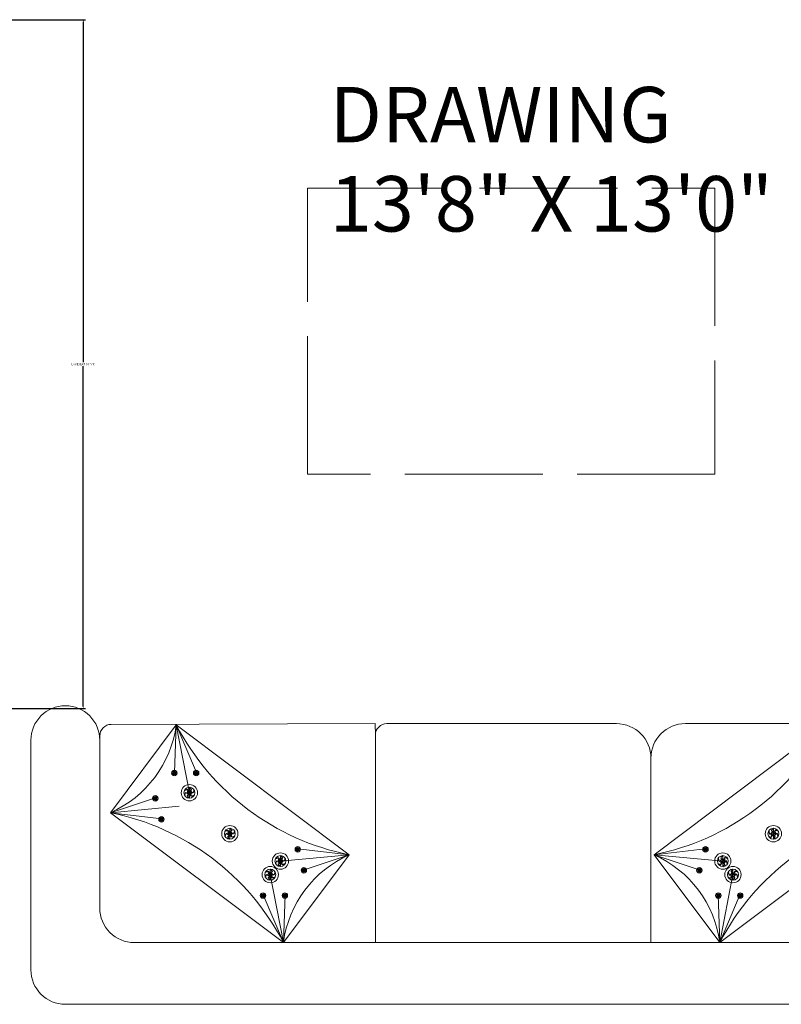
# Model space of a CAD drawing. Units: inches. Extents: x -61 to 1599, y -1316 to 257.
# Tile 198 of 204: x 1396 to 1463, y -164 to -78. Entities that reach past the tile are written whole.
import ezdxf

# ---------------------------------------------------------------- set-up
doc = ezdxf.new("R2010")
doc.units = ezdxf.units.IN
doc.header["$MEASUREMENT"] = 0
doc.linetypes.add('ACAD_ISO02W100', pattern=[15, 12, -3])
for name, color, linetype, lineweight in [('A-ANNO-DIMS', 2, 'Continuous', 18), ('A-AREA-IDEN', 1, 'Continuous', 18), ('A-FURN-LOW', 83, 'ACAD_ISO02W100', 18), ('FURNITURE', 83, 'Continuous', 18)]:
    doc.layers.add(name, color=color, linetype=linetype, lineweight=lineweight)
doc.layers.add('FUR', color=83, linetype='Continuous')
doc.styles.get("Standard").update_dxf_attribs({"font": 'arial.ttf'})
doc.dimstyles.get("Standard").update_dxf_attribs({"dimtxt": 0.18, "dimasz": 0.18, "dimexe": 0.18, "dimexo": 0.0625, "dimgap": 0.09, "dimtad": 0, "dimtih": 1, "dimtoh": 1, "dimdec": 0, "dimzin": 0, "dimdsep": 46, "dimlunit": 3, "dimtxsty": 'Standard', "dimcen": 0.09, "dimadec": 0, "dimazin": 0, "dimtfac": 1, "dimtdec": 0, "dimtofl": 0, "dimtmove": 0, "dimatfit": 3, "dimfxl": 1, "dimtolj": 1, "dimtzin": 0, "dimarcsym": 0})

# ---------------------------------------------------------------- blocks, each defined once
blk = doc.blocks.new('*U152')
at = {"layer": 'FUR'}
blk.add_open_spline([(0.005, 0.08), (-0.03, 0.048), (-0.098, -0.015), (0.075, -0.018), (0.024, -0.063), (0.005, -0.08)], degree=3, knots=[0, 0, 0, 0, 0.0954578, 0.1898773, 0.2470677, 0.2470677, 0.2470677, 0.2470677], dxfattribs=at)
blk = doc.blocks.new('*U153')
at = {"layer": 'FUR', "transparency": 16777216}
for p, rotation in [((222.173, -79.977), 60), ((222.178, -80.056), 120), ((222.25, -80.092), 180), ((222.312, -79.968), 300), ((222.317, -80.048), 240)]:
    blk.add_blockref('*U152', p, dxfattribs=dict(at, rotation=rotation))
blk.add_blockref('*U152', (222.24, -79.932), dxfattribs=at)
blk = doc.blocks.new('*U154')
at = {"layer": 'FUR'}
blk.add_open_spline([(0.005, 0.08), (-0.03, 0.048), (-0.098, -0.015), (0.075, -0.018), (0.024, -0.063), (0.005, -0.08)], degree=3, knots=[0, 0, 0, 0, 0.0954578, 0.1898773, 0.2470677, 0.2470677, 0.2470677, 0.2470677], dxfattribs=at)
blk = doc.blocks.new('*U155')
at = {"layer": 'FUR', "transparency": 16777216}
for p, rotation in [((222.173, -79.977), 60), ((222.178, -80.056), 120), ((222.25, -80.092), 180), ((222.312, -79.968), 300), ((222.317, -80.048), 240)]:
    blk.add_blockref('*U154', p, dxfattribs=dict(at, rotation=rotation))
blk.add_blockref('*U154', (222.24, -79.932), dxfattribs=at)
blk = doc.blocks.new('*U148')
at = {"layer": 'FUR'}
blk.add_open_spline([(0.005, 0.08), (-0.03, 0.048), (-0.098, -0.015), (0.075, -0.018), (0.024, -0.063), (0.005, -0.08)], degree=3, knots=[0, 0, 0, 0, 0.0954578, 0.1898773, 0.2470677, 0.2470677, 0.2470677, 0.2470677], dxfattribs=at)
blk = doc.blocks.new('*U149')
at = {"layer": 'FUR', "transparency": 16777216}
for p, rotation in [((222.173, -79.977), 60), ((222.178, -80.056), 120), ((222.25, -80.092), 180), ((222.312, -79.968), 300), ((222.317, -80.048), 240)]:
    blk.add_blockref('*U148', p, dxfattribs=dict(at, rotation=rotation))
blk.add_blockref('*U148', (222.24, -79.932), dxfattribs=at)
blk = doc.blocks.new('*U128')
at = {"layer": 'FUR'}
blk.add_open_spline([(0.015, 0.238), (-0.088, 0.143), (-0.292, -0.045), (0.224, -0.053), (0.072, -0.187), (0.015, -0.238)], degree=3, knots=[0, 0, 0, 0, 0.2846533, 0.5662105, 0.736751, 0.736751, 0.736751, 0.736751], dxfattribs=at)
blk = doc.blocks.new('*U129')
at = {"layer": 'FUR', "transparency": 16777216}
for p, rotation in [((662.517, -238.489), 60), ((662.929, -238.463), 300), ((662.531, -238.727), 120), ((662.745, -238.833), 180), ((662.944, -238.702), 240)]:
    blk.add_blockref('*U128', p, dxfattribs=dict(at, rotation=rotation))
blk.add_blockref('*U128', (662.716, -238.357), dxfattribs=at)
blk = doc.blocks.new('*U150')
at = {"layer": 'FUR'}
blk.add_open_spline([(0.005, 0.08), (-0.03, 0.048), (-0.098, -0.015), (0.075, -0.018), (0.024, -0.063), (0.005, -0.08)], degree=3, knots=[0, 0, 0, 0, 0.0954578, 0.1898773, 0.2470677, 0.2470677, 0.2470677, 0.2470677], dxfattribs=at)
blk = doc.blocks.new('*U151')
at = {"layer": 'FUR', "transparency": 16777216}
for p, rotation in [((222.173, -79.977), 60), ((222.178, -80.056), 120), ((222.25, -80.092), 180), ((222.312, -79.968), 300), ((222.317, -80.048), 240)]:
    blk.add_blockref('*U150', p, dxfattribs=dict(at, rotation=rotation))
blk.add_blockref('*U150', (222.24, -79.932), dxfattribs=at)
blk = doc.blocks.new('*U132')
at = {"layer": 'FUR'}
blk.add_open_spline([(0.015, 0.238), (-0.088, 0.143), (-0.292, -0.045), (0.224, -0.053), (0.072, -0.187), (0.015, -0.238)], degree=3, knots=[0, 0, 0, 0, 0.2846533, 0.5662105, 0.736751, 0.736751, 0.736751, 0.736751], dxfattribs=at)
blk = doc.blocks.new('*U133')
at = {"layer": 'FUR', "transparency": 16777216}
for p, rotation in [((662.517, -238.489), 60), ((662.929, -238.463), 300), ((662.531, -238.727), 120), ((662.745, -238.833), 180), ((662.944, -238.702), 240)]:
    blk.add_blockref('*U132', p, dxfattribs=dict(at, rotation=rotation))
blk.add_blockref('*U132', (662.716, -238.357), dxfattribs=at)
blk = doc.blocks.new('*U124')
at = {"layer": 'FUR'}
blk.add_open_spline([(0.005, 0.08), (-0.03, 0.048), (-0.098, -0.015), (0.075, -0.018), (0.024, -0.063), (0.005, -0.08)], degree=3, knots=[0, 0, 0, 0, 0.0954578, 0.1898773, 0.2470677, 0.2470677, 0.2470677, 0.2470677], dxfattribs=at)
blk = doc.blocks.new('*U125')
at = {"layer": 'FUR', "transparency": 16777216}
for p, rotation in [((222.173, -79.977), 60), ((222.178, -80.056), 120), ((222.25, -80.092), 180), ((222.312, -79.968), 300), ((222.317, -80.048), 240)]:
    blk.add_blockref('*U124', p, dxfattribs=dict(at, rotation=rotation))
blk.add_blockref('*U124', (222.24, -79.932), dxfattribs=at)
blk = doc.blocks.new('*U134')
at = {"layer": 'FUR'}
blk.add_open_spline([(0.015, 0.238), (-0.088, 0.143), (-0.292, -0.045), (0.224, -0.053), (0.072, -0.187), (0.015, -0.238)], degree=3, knots=[0, 0, 0, 0, 0.2846533, 0.5662105, 0.736751, 0.736751, 0.736751, 0.736751], dxfattribs=at)
blk = doc.blocks.new('*U123')
at = {"layer": 'FUR', "transparency": 16777216}
for p, rotation in [((662.517, -238.489), 60), ((662.929, -238.463), 300), ((662.531, -238.727), 120), ((662.745, -238.833), 180), ((662.944, -238.702), 240)]:
    blk.add_blockref('*U134', p, dxfattribs=dict(at, rotation=rotation))
blk.add_blockref('*U134', (662.716, -238.357), dxfattribs=at)
blk = doc.blocks.new('*U130')
at = {"layer": 'FUR'}
blk.add_open_spline([(0.015, 0.238), (-0.088, 0.143), (-0.292, -0.045), (0.224, -0.053), (0.072, -0.187), (0.015, -0.238)], degree=3, knots=[0, 0, 0, 0, 0.2846533, 0.5662105, 0.736751, 0.736751, 0.736751, 0.736751], dxfattribs=at)
blk = doc.blocks.new('*U131')
at = {"layer": 'FUR', "transparency": 16777216}
for p, rotation in [((662.517, -238.489), 60), ((662.929, -238.463), 300), ((662.531, -238.727), 120), ((662.745, -238.833), 180), ((662.944, -238.702), 240)]:
    blk.add_blockref('*U130', p, dxfattribs=dict(at, rotation=rotation))
blk.add_blockref('*U130', (662.716, -238.357), dxfattribs=at)
blk = doc.blocks.new('*U126')
at = {"layer": 'FUR'}
blk.add_open_spline([(0.005, 0.08), (-0.03, 0.048), (-0.098, -0.015), (0.075, -0.018), (0.024, -0.063), (0.005, -0.08)], degree=3, knots=[0, 0, 0, 0, 0.0954578, 0.1898773, 0.2470677, 0.2470677, 0.2470677, 0.2470677], dxfattribs=at)
blk = doc.blocks.new('*U127')
at = {"layer": 'FUR', "transparency": 16777216}
for p, rotation in [((222.173, -79.977), 60), ((222.178, -80.056), 120), ((222.25, -80.092), 180), ((222.312, -79.968), 300), ((222.317, -80.048), 240)]:
    blk.add_blockref('*U126', p, dxfattribs=dict(at, rotation=rotation))
blk.add_blockref('*U126', (222.24, -79.932), dxfattribs=at)
blk = doc.blocks.new('*U146')
at = {"layer": 'FUR'}
blk.add_open_spline([(0.005, 0.08), (-0.03, 0.048), (-0.098, -0.015), (0.075, -0.018), (0.024, -0.063), (0.005, -0.08)], degree=3, knots=[0, 0, 0, 0, 0.0954578, 0.1898773, 0.2470677, 0.2470677, 0.2470677, 0.2470677], dxfattribs=at)
blk = doc.blocks.new('*U147')
at = {"layer": 'FUR', "transparency": 16777216}
for p, rotation in [((222.173, -79.977), 60), ((222.178, -80.056), 120), ((222.25, -80.092), 180), ((222.312, -79.968), 300), ((222.317, -80.048), 240)]:
    blk.add_blockref('*U146', p, dxfattribs=dict(at, rotation=rotation))
blk.add_blockref('*U146', (222.24, -79.932), dxfattribs=at)
blk = doc.blocks.new('*U144')
at = {"layer": 'FUR'}
blk.add_open_spline([(0.005, 0.08), (-0.03, 0.048), (-0.098, -0.015), (0.075, -0.018), (0.024, -0.063), (0.005, -0.08)], degree=3, knots=[0, 0, 0, 0, 0.0954578, 0.1898773, 0.2470677, 0.2470677, 0.2470677, 0.2470677], dxfattribs=at)
blk = doc.blocks.new('*U145')
at = {"layer": 'FUR', "transparency": 16777216}
for p, rotation in [((222.173, -79.977), 60), ((222.178, -80.056), 120), ((222.25, -80.092), 180), ((222.312, -79.968), 300), ((222.317, -80.048), 240)]:
    blk.add_blockref('*U144', p, dxfattribs=dict(at, rotation=rotation))
blk.add_blockref('*U144', (222.24, -79.932), dxfattribs=at)
blk = doc.blocks.new('*U114')
at = {"layer": 'FUR'}
blk.add_open_spline([(0.005, 0.08), (-0.03, 0.048), (-0.098, -0.015), (0.075, -0.018), (0.024, -0.063), (0.005, -0.08)], degree=3, knots=[0, 0, 0, 0, 0.0954578, 0.1898773, 0.2470677, 0.2470677, 0.2470677, 0.2470677], dxfattribs=at)
blk = doc.blocks.new('*U115')
at = {"layer": 'FUR', "transparency": 16777216}
for p, rotation in [((222.173, -79.977), 60), ((222.178, -80.056), 120), ((222.25, -80.092), 180), ((222.312, -79.968), 300), ((222.317, -80.048), 240)]:
    blk.add_blockref('*U114', p, dxfattribs=dict(at, rotation=rotation))
blk.add_blockref('*U114', (222.24, -79.932), dxfattribs=at)
blk = doc.blocks.new('*U116')
at = {"layer": 'FUR'}
blk.add_open_spline([(0.005, 0.08), (-0.03, 0.048), (-0.098, -0.015), (0.075, -0.018), (0.024, -0.063), (0.005, -0.08)], degree=3, knots=[0, 0, 0, 0, 0.0954578, 0.1898773, 0.2470677, 0.2470677, 0.2470677, 0.2470677], dxfattribs=at)
blk = doc.blocks.new('*U117')
at = {"layer": 'FUR', "transparency": 16777216}
for p, rotation in [((222.173, -79.977), 60), ((222.178, -80.056), 120), ((222.25, -80.092), 180), ((222.312, -79.968), 300), ((222.317, -80.048), 240)]:
    blk.add_blockref('*U116', p, dxfattribs=dict(at, rotation=rotation))
blk.add_blockref('*U116', (222.24, -79.932), dxfattribs=at)
blk = doc.blocks.new('*U112')
at = {"layer": 'FUR'}
blk.add_open_spline([(0.005, 0.08), (-0.03, 0.048), (-0.098, -0.015), (0.075, -0.018), (0.024, -0.063), (0.005, -0.08)], degree=3, knots=[0, 0, 0, 0, 0.0954578, 0.1898773, 0.2470677, 0.2470677, 0.2470677, 0.2470677], dxfattribs=at)
blk = doc.blocks.new('*U113')
at = {"layer": 'FUR', "transparency": 16777216}
for p, rotation in [((222.173, -79.977), 60), ((222.178, -80.056), 120), ((222.25, -80.092), 180), ((222.312, -79.968), 300), ((222.317, -80.048), 240)]:
    blk.add_blockref('*U112', p, dxfattribs=dict(at, rotation=rotation))
blk.add_blockref('*U112', (222.24, -79.932), dxfattribs=at)
blk = doc.blocks.new('*U142')
at = {"layer": 'FUR'}
blk.add_open_spline([(0.015, 0.238), (-0.088, 0.143), (-0.292, -0.045), (0.224, -0.053), (0.072, -0.187), (0.015, -0.238)], degree=3, knots=[0, 0, 0, 0, 0.2846533, 0.5662105, 0.736751, 0.736751, 0.736751, 0.736751], dxfattribs=at)
blk = doc.blocks.new('*U143')
at = {"layer": 'FUR', "transparency": 16777216}
for p, rotation in [((662.517, -238.489), 60), ((662.929, -238.463), 300), ((662.531, -238.727), 120), ((662.745, -238.833), 180), ((662.944, -238.702), 240)]:
    blk.add_blockref('*U142', p, dxfattribs=dict(at, rotation=rotation))
blk.add_blockref('*U142', (662.716, -238.357), dxfattribs=at)
blk = doc.blocks.new('*U158')
at = {"layer": 'FUR'}
blk.add_open_spline([(0.015, 0.238), (-0.088, 0.143), (-0.292, -0.045), (0.224, -0.053), (0.072, -0.187), (0.015, -0.238)], degree=3, knots=[0, 0, 0, 0, 0.2846533, 0.5662105, 0.736751, 0.736751, 0.736751, 0.736751], dxfattribs=at)
blk = doc.blocks.new('*U109')
at = {"layer": 'FUR', "transparency": 16777216}
for p, rotation in [((662.517, -238.489), 60), ((662.929, -238.463), 300), ((662.531, -238.727), 120), ((662.745, -238.833), 180), ((662.944, -238.702), 240)]:
    blk.add_blockref('*U158', p, dxfattribs=dict(at, rotation=rotation))
blk.add_blockref('*U158', (662.716, -238.357), dxfattribs=at)
blk = doc.blocks.new('*U110')
at = {"layer": 'FUR'}
blk.add_open_spline([(0.005, 0.08), (-0.03, 0.048), (-0.098, -0.015), (0.075, -0.018), (0.024, -0.063), (0.005, -0.08)], degree=3, knots=[0, 0, 0, 0, 0.0954578, 0.1898773, 0.2470677, 0.2470677, 0.2470677, 0.2470677], dxfattribs=at)
blk = doc.blocks.new('*U111')
at = {"layer": 'FUR', "transparency": 16777216}
for p, rotation in [((222.173, -79.977), 60), ((222.178, -80.056), 120), ((222.25, -80.092), 180), ((222.312, -79.968), 300), ((222.317, -80.048), 240)]:
    blk.add_blockref('*U110', p, dxfattribs=dict(at, rotation=rotation))
blk.add_blockref('*U110', (222.24, -79.932), dxfattribs=at)
blk = doc.blocks.new('*U156')
at = {"layer": 'FUR'}
blk.add_open_spline([(0.015, 0.238), (-0.088, 0.143), (-0.292, -0.045), (0.224, -0.053), (0.072, -0.187), (0.015, -0.238)], degree=3, knots=[0, 0, 0, 0, 0.2846533, 0.5662105, 0.736751, 0.736751, 0.736751, 0.736751], dxfattribs=at)
blk = doc.blocks.new('*U157')
at = {"layer": 'FUR', "transparency": 16777216}
for p, rotation in [((662.517, -238.489), 60), ((662.929, -238.463), 300), ((662.531, -238.727), 120), ((662.745, -238.833), 180), ((662.944, -238.702), 240)]:
    blk.add_blockref('*U156', p, dxfattribs=dict(at, rotation=rotation))
blk.add_blockref('*U156', (662.716, -238.357), dxfattribs=at)
blk = doc.blocks.new('*U120')
at = {"layer": 'FUR'}
blk.add_open_spline([(0.005, 0.08), (-0.03, 0.048), (-0.098, -0.015), (0.075, -0.018), (0.024, -0.063), (0.005, -0.08)], degree=3, knots=[0, 0, 0, 0, 0.0954578, 0.1898773, 0.2470677, 0.2470677, 0.2470677, 0.2470677], dxfattribs=at)
blk = doc.blocks.new('*U121')
at = {"layer": 'FUR', "transparency": 16777216}
for p, rotation in [((222.173, -79.977), 60), ((222.178, -80.056), 120), ((222.25, -80.092), 180), ((222.312, -79.968), 300), ((222.317, -80.048), 240)]:
    blk.add_blockref('*U120', p, dxfattribs=dict(at, rotation=rotation))
blk.add_blockref('*U120', (222.24, -79.932), dxfattribs=at)
blk = doc.blocks.new('*U140')
at = {"layer": 'FUR'}
blk.add_open_spline([(0.015, 0.238), (-0.088, 0.143), (-0.292, -0.045), (0.224, -0.053), (0.072, -0.187), (0.015, -0.238)], degree=3, knots=[0, 0, 0, 0, 0.2846533, 0.5662105, 0.736751, 0.736751, 0.736751, 0.736751], dxfattribs=at)
blk = doc.blocks.new('*U141')
at = {"layer": 'FUR', "transparency": 16777216}
for p, rotation in [((662.517, -238.489), 60), ((662.929, -238.463), 300), ((662.531, -238.727), 120), ((662.745, -238.833), 180), ((662.944, -238.702), 240)]:
    blk.add_blockref('*U140', p, dxfattribs=dict(at, rotation=rotation))
blk.add_blockref('*U140', (662.716, -238.357), dxfattribs=at)
blk = doc.blocks.new('*U135')
at = {"layer": 'FUR'}
blk.add_open_spline([(0.015, 0.238), (-0.088, 0.143), (-0.292, -0.045), (0.224, -0.053), (0.072, -0.187), (0.015, -0.238)], degree=3, knots=[0, 0, 0, 0, 0.2846533, 0.5662105, 0.736751, 0.736751, 0.736751, 0.736751], dxfattribs=at)
blk = doc.blocks.new('*U136')
at = {"layer": 'FUR', "transparency": 16777216}
for p, rotation in [((662.517, -238.489), 60), ((662.929, -238.463), 300), ((662.531, -238.727), 120), ((662.745, -238.833), 180), ((662.944, -238.702), 240)]:
    blk.add_blockref('*U135', p, dxfattribs=dict(at, rotation=rotation))
blk.add_blockref('*U135', (662.716, -238.357), dxfattribs=at)
blk = doc.blocks.new('*U118')
at = {"layer": 'FUR'}
blk.add_open_spline([(0.005, 0.08), (-0.03, 0.048), (-0.098, -0.015), (0.075, -0.018), (0.024, -0.063), (0.005, -0.08)], degree=3, knots=[0, 0, 0, 0, 0.0954578, 0.1898773, 0.2470677, 0.2470677, 0.2470677, 0.2470677], dxfattribs=at)
blk = doc.blocks.new('*U119')
at = {"layer": 'FUR', "transparency": 16777216}
for p, rotation in [((222.173, -79.977), 60), ((222.178, -80.056), 120), ((222.25, -80.092), 180), ((222.312, -79.968), 300), ((222.317, -80.048), 240)]:
    blk.add_blockref('*U118', p, dxfattribs=dict(at, rotation=rotation))
blk.add_blockref('*U118', (222.24, -79.932), dxfattribs=at)
blk = doc.blocks.new('*U138')
at = {"layer": 'FUR'}
blk.add_open_spline([(0.005, 0.08), (-0.03, 0.048), (-0.098, -0.015), (0.075, -0.018), (0.024, -0.063), (0.005, -0.08)], degree=3, knots=[0, 0, 0, 0, 0.0954578, 0.1898773, 0.2470677, 0.2470677, 0.2470677, 0.2470677], dxfattribs=at)
blk = doc.blocks.new('*U139')
at = {"layer": 'FUR', "transparency": 16777216}
for p, rotation in [((222.173, -79.977), 60), ((222.178, -80.056), 120), ((222.25, -80.092), 180), ((222.312, -79.968), 300), ((222.317, -80.048), 240)]:
    blk.add_blockref('*U138', p, dxfattribs=dict(at, rotation=rotation))
blk.add_blockref('*U138', (222.24, -79.932), dxfattribs=at)
blk = doc.blocks.new('*U122')
at = {"layer": 'FUR'}
blk.add_open_spline([(0.005, 0.08), (-0.03, 0.048), (-0.098, -0.015), (0.075, -0.018), (0.024, -0.063), (0.005, -0.08)], degree=3, knots=[0, 0, 0, 0, 0.0954578, 0.1898773, 0.2470677, 0.2470677, 0.2470677, 0.2470677], dxfattribs=at)
blk = doc.blocks.new('*U137')
at = {"layer": 'FUR', "transparency": 16777216}
for p, rotation in [((222.173, -79.977), 60), ((222.178, -80.056), 120), ((222.25, -80.092), 180), ((222.312, -79.968), 300), ((222.317, -80.048), 240)]:
    blk.add_blockref('*U122', p, dxfattribs=dict(at, rotation=rotation))
blk.add_blockref('*U122', (222.24, -79.932), dxfattribs=at)
blk = doc.blocks.new('SOFA-THREE-SEAT')
for p, q in [((30, 24.442), (6.996, 24.38)), ((12.664, 24.333), (12.509, 20.192)), ((12.664, 24.333), (13.805, 18.423)), ((12.664, 24.333), (14.414, 20.192)), ((30, 23.442), (29.997, 24.442)), ((51, 24.442), (31, 24.442)), ((78.369, 24.442), (57, 24.442)), ((69.336, 24.333), (67.586, 20.192)), ((69.336, 24.333), (68.194, 18.423)), ((69.336, 24.333), (69.49, 20.192)), ((6, 23), (5.999, 23.377)), ((30, 23.442), (30, 5.382)), ((54, 21.442), (54, 5.382)), ((54, 21.442), (54, 21.442)), ((12.49, 20.139), (12.49, 20.299)), ((12.49, 20.139), (12.49, 19.979)), ((14.394, 20.139), (14.394, 20.299)), ((14.394, 20.139), (14.394, 19.979)), ((67.605, 20.139), (67.605, 20.299)), ((67.605, 20.139), (67.605, 19.979)), ((69.509, 20.139), (69.509, 20.299)), ((69.509, 20.139), (69.509, 19.979)), ((13.805, 18.423), (13.805, 18.899)), ((68.194, 18.423), (68.194, 18.899)), ((10.84, 17.94), (10.84, 18.1)), ((13.805, 18.423), (13.805, 17.946)), ((68.194, 18.423), (68.194, 17.946)), ((71.159, 17.94), (71.159, 18.1)), ((6.926, 16.687), (10.859, 17.993)), ((6.926, 16.687), (12.92, 17.243)), ((10.84, 17.94), (10.84, 17.78)), ((69.079, 17.243), (69.079, 17.719)), ((75.074, 16.687), (69.079, 17.243)), ((69.079, 17.243), (69.079, 16.766)), ((75.074, 16.687), (71.14, 17.993)), ((71.159, 17.94), (71.159, 17.78)), ((6.926, 16.687), (11.391, 16.164)), ((75.074, 16.687), (70.608, 16.164)), ((11.372, 16.112), (11.372, 16.272)), ((11.372, 16.112), (11.372, 15.952)), ((70.627, 16.112), (70.627, 16.272)), ((70.627, 16.112), (70.627, 15.952)), ((17.327, 14.857), (17.327, 15.334)), ((17.327, 14.857), (17.327, 14.381)), ((64.672, 14.857), (64.672, 15.334)), ((64.672, 14.857), (64.672, 14.381)), ((27.729, 13.028), (21.735, 12.472)), ((21.735, 12.472), (21.735, 12.949)), ((23.243, 13.498), (23.243, 13.658)), ((23.243, 13.498), (23.243, 13.338)), ((27.729, 13.028), (23.263, 13.551)), ((27.729, 13.028), (23.795, 11.722)), ((54.271, 13.028), (58.736, 13.551)), ((54.271, 13.028), (60.265, 12.472)), ((54.271, 13.028), (58.204, 11.722)), ((58.756, 13.498), (58.756, 13.658)), ((58.756, 13.498), (58.756, 13.338)), ((60.265, 12.472), (60.265, 12.949)), ((21.735, 12.472), (21.735, 11.996)), ((60.265, 12.472), (60.265, 11.996)), ((20.849, 11.292), (20.849, 11.769)), ((21.991, 5.382), (20.849, 11.292)), ((20.849, 11.292), (20.849, 10.816)), ((23.776, 11.67), (23.776, 11.83)), ((23.776, 11.67), (23.776, 11.51)), ((58.224, 11.67), (58.224, 11.83)), ((58.224, 11.67), (58.224, 11.51)), ((60.009, 5.382), (61.15, 11.292)), ((61.15, 11.292), (61.15, 11.769)), ((61.15, 11.292), (61.15, 10.816)), ((20.221, 9.471), (20.221, 9.631)), ((20.221, 9.471), (20.221, 9.311)), ((21.991, 5.382), (20.241, 9.523)), ((21.991, 5.382), (22.145, 9.523)), ((22.125, 9.471), (22.125, 9.631)), ((22.125, 9.471), (22.125, 9.311)), ((60.009, 5.382), (59.854, 9.523)), ((59.874, 9.471), (59.874, 9.631)), ((59.874, 9.471), (59.874, 9.311)), ((60.009, 5.382), (61.759, 9.523)), ((61.778, 9.471), (61.778, 9.631)), ((61.778, 9.471), (61.778, 9.311))]:
    blk.add_line(p, q)
blk.add_lwpolyline([(78, 8.382), (78, 23, -0.414214), (81, 26), (81, 26, -0.414214), (84, 23), (84, 3, -0.414214), (81, 0), (3, 0, -0.414214), (0, 3), (0, 23, -0.414214), (3, 26), (3, 26, -0.414214), (6, 23), (6, 8.382, 0.414214), (9, 5.382), (75, 5.382, 0.414214)], format="xyb", close=True)
for points in [[(27.729, 13.028), (12.664, 24.333), (6.926, 16.687), (21.991, 5.382)], [(54.271, 13.028), (69.336, 24.333), (75.074, 16.687), (60.009, 5.382)]]:
    blk.add_lwpolyline(points, close=True)
for centre, radius in [((12.49, 20.139), 0.238), ((12.49, 20.139), 0.16), ((14.394, 20.139), 0.238), ((14.394, 20.139), 0.16), ((67.605, 20.139), 0.238), ((67.605, 20.139), 0.16), ((69.509, 20.139), 0.238), ((69.509, 20.139), 0.16), ((13.805, 18.423), 0.71), ((13.805, 18.423), 0.476), ((68.194, 18.423), 0.71), ((68.194, 18.423), 0.476), ((10.84, 17.94), 0.238), ((10.84, 17.94), 0.16), ((71.159, 17.94), 0.238), ((71.159, 17.94), 0.16), ((69.079, 17.243), 0.71), ((69.079, 17.243), 0.476), ((11.372, 16.112), 0.238), ((70.627, 16.112), 0.238), ((11.372, 16.112), 0.16), ((17.327, 14.857), 0.71), ((64.672, 14.857), 0.71), ((70.627, 16.112), 0.16), ((17.327, 14.857), 0.476), ((64.672, 14.857), 0.476), ((23.243, 13.498), 0.238), ((58.756, 13.498), 0.238), ((21.735, 12.472), 0.71), ((21.735, 12.472), 0.476), ((23.243, 13.498), 0.16), ((58.756, 13.498), 0.16), ((60.265, 12.472), 0.71), ((60.265, 12.472), 0.476), ((20.849, 11.292), 0.71), ((20.849, 11.292), 0.476), ((23.776, 11.67), 0.238), ((23.776, 11.67), 0.16), ((58.224, 11.67), 0.238), ((58.224, 11.67), 0.16), ((61.15, 11.292), 0.71), ((61.15, 11.292), 0.476), ((20.221, 9.471), 0.238), ((20.221, 9.471), 0.16), ((22.125, 9.471), 0.238), ((22.125, 9.471), 0.16), ((59.874, 9.471), 0.238), ((59.874, 9.471), 0.16), ((61.778, 9.471), 0.238), ((61.778, 9.471), 0.16)]:
    blk.add_circle(centre, radius)
for centre, radius, start, end in [((6.999, 23.38), 1, 90.15417, 180.15417), ((2.937, 25.656), 9.816, 293.97422, 352.25297), ((31.951, 34.345), 21.731, 207.43163, 258.79556), ((31, 23.442), 1, 89.99998, 179.99998), ((51, 21.442), 3, 359.99998, 89.99998), ((57, 21.442), 3, 90, 180.00002), ((50.048, 34.345), 21.731, 281.20444, 332.56837), ((79.062, 25.656), 9.816, 187.74703, 246.02578), ((2.703, -4.63), 21.731, 27.43163, 78.79556), ((79.296, -4.63), 21.731, 101.20444, 152.56837), ((31.717, 4.059), 9.816, 113.97422, 172.25297), ((50.282, 4.059), 9.816, 7.74703, 66.02578)]:
    blk.add_arc(centre, radius, start, end)
at = {"xscale": -1, "rotation": 180}
for name, p in [('*U149', (-209.755, -59.873)), ('*U151', (-207.851, -59.873)), ('*U129', (-648.925, -220.172)), ('*U153', (-211.405, -62.072)), ('*U155', (-210.873, -63.9)), ('*U133', (-645.403, -223.738)), ('*U131', (-640.996, -226.123)), ('*U147', (-199.001, -66.514)), ('*U123', (-641.881, -227.303)), ('*U145', (-198.469, -68.342)), ('*U125', (-202.024, -70.541)), ('*U127', (-200.12, -70.541))]:
    blk.add_blockref(name, p, dxfattribs=at)
at = {"rotation": 180}
for name, p in [('*U121', (289.85, -59.873)), ('*U119', (291.754, -59.873)), ('*U141', (730.924, -220.172)), ('*U137', (293.404, -62.072)), ('*U136', (731.81, -221.352)), ('*U139', (292.872, -63.9)), ('*U157', (727.402, -223.738)), ('*U117', (281.001, -66.514)), ('*U143', (722.995, -226.123)), ('*U115', (280.469, -68.342)), ('*U109', (723.88, -227.303)), ('*U113', (282.119, -70.541)), ('*U111', (284.023, -70.541))]:
    blk.add_blockref(name, p, dxfattribs=at)
blk = doc.blocks.new('*D636')
at = {"layer": 'A-ANNO-DIMS', "color": 0, "lineweight": -2, "transparency": 16777216}
for p, q in [((1393.015, -78.383), (1402.132, -78.383)), ((1401.952, -78.563), (1401.952, -108.2)), ((1401.952, -138.203), (1401.952, -108.566)), ((1393.015, -138.383), (1402.132, -138.383))]:
    blk.add_line(p, q, dxfattribs=at)
at = {"layer": 'A-ANNO-DIMS', "color": 0, "transparency": 16777216}
for points in [[(1401.922, -78.563), (1401.982, -78.563), (1401.952, -78.383)], [(1401.922, -138.203), (1401.982, -138.203), (1401.952, -138.383)]]:
    blk.add_solid(points, dxfattribs=at)
at = {"layer": 'DEFPOINTS', "color": 0, "transparency": 16777216}
for p in [(1392.952, -78.383), (1401.952, -78.383), (1392.952, -138.383)]:
    blk.add_point(p, dxfattribs=at)
at = {"layer": 'A-ANNO-DIMS', "color": 0, "transparency": 16777216, "insert": (1401.952, -108.383), "char_height": 0.18, "attachment_point": 5}
blk.add_mtext('\\A1;LOVESEAT 60 TYP.', dxfattribs=at)

msp = doc.modelspace()

# ---------------------------------------------------------------- linework, layer by layer
at = {"layer": 'A-FURN-LOW'}
msp.add_lwpolyline([(1456.9662, -117.9559), (1421.4644, -117.9559), (1421.4644, -93.0522), (1456.9662, -93.0522)], close=True, dxfattribs=at)

# ---------------------------------------------------------------- block references
at = {"layer": 'FURNITURE'}
msp.add_blockref('SOFA-THREE-SEAT', (1397.3851, -164.1303), dxfattribs=at)

# ---------------------------------------------------------------- texts
at = {"layer": 'A-AREA-IDEN'}
for s, height, p in [('DRAWING', 4.8321, (1423.4206, -89.0692)), ('13\'8" X 13\'0"', 4.832098, (1423.4206, -96.8315))]:
    msp.add_text(s, height=height, dxfattribs=at).set_placement(p)

# ---------------------------------------------------------------- dimensions: what is measured, and where the dimension line sits
at = {"layer": 'A-ANNO-DIMS'}
dim = msp.add_linear_dim(base=(1401.9522, -78.3832), p1=(1392.9522, -138.3833), p2=(1392.9522, -78.3832), angle=90, text='LOVESEAT <> TYP.', dimstyle='Standard', override={"dimdec": 0, "dimlfac": 1, "dimrnd": 0, "dimzin": 0, "dimdsep": 46, "dimlunit": 2}, dxfattribs=at)
dim.commit()
dim.dimension.update_dxf_attribs({"geometry": '*D636', "text_midpoint": (1401.9522, -108.3832)})

doc.saveas('drawing.dxf')
